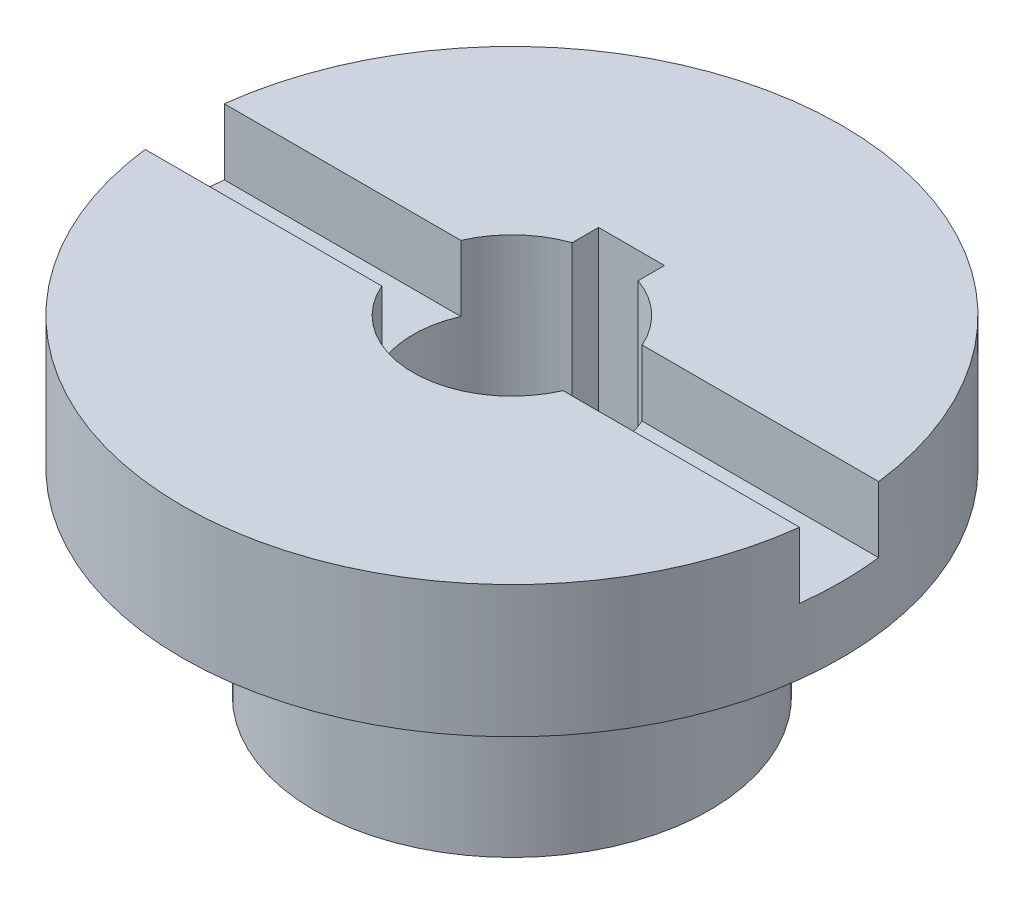
ISO-10303-21;
HEADER;
FILE_DESCRIPTION(('STEP AP214'),'2;1');
FILE_NAME('part.step','',(''),(''),'','','');
FILE_SCHEMA(('AUTOMOTIVE_DESIGN { 1 0 10303 214 1 1 1 1 }'));
ENDSEC;
DATA;
#1=APPLICATION_CONTEXT('core data for automotive mechanical design processes');
#2=APPLICATION_PROTOCOL_DEFINITION('international standard','automotive_design',2000,#1);
#3=PRODUCT_CONTEXT('',#1,'mechanical');
#4=PRODUCT('Part','Part','',(#3));
#5=PRODUCT_RELATED_PRODUCT_CATEGORY('part','',(#4));
#6=PRODUCT_DEFINITION_FORMATION('','',#4);
#7=PRODUCT_DEFINITION_CONTEXT('part definition',#1,'design');
#8=PRODUCT_DEFINITION('design','',#6,#7);
#9=PRODUCT_DEFINITION_SHAPE('','',#8);
#10=(LENGTH_UNIT() NAMED_UNIT(*) SI_UNIT(.MILLI.,.METRE.));
#11=(NAMED_UNIT(*) PLANE_ANGLE_UNIT() SI_UNIT($,.RADIAN.));
#12=(NAMED_UNIT(*) SI_UNIT($,.STERADIAN.) SOLID_ANGLE_UNIT());
#13=UNCERTAINTY_MEASURE_WITH_UNIT(LENGTH_MEASURE(1.E-05),#10,'distance_accuracy_value','');
#14=(GEOMETRIC_REPRESENTATION_CONTEXT(3) GLOBAL_UNCERTAINTY_ASSIGNED_CONTEXT((#13)) GLOBAL_UNIT_ASSIGNED_CONTEXT((#10,
#11,#12)) REPRESENTATION_CONTEXT('',''));
#15=CARTESIAN_POINT('',(0.,0.,0.));
#16=DIRECTION('',(0.,0.,1.));
#17=DIRECTION('',(1.,0.,0.));
#18=AXIS2_PLACEMENT_3D('',#15,#16,#17);
#19=CARTESIAN_POINT('',(0.,0.,0.));
#20=DIRECTION('',(0.,-1.,0.));
#21=DIRECTION('',(0.,0.,-1.));
#22=AXIS2_PLACEMENT_3D('',#19,#20,#21);
#23=PLANE('',#22);
#24=CARTESIAN_POINT('',(0.,0.,0.));
#25=DIRECTION('',(0.,1.,0.));
#26=DIRECTION('',(0.,0.,1.));
#27=AXIS2_PLACEMENT_3D('',#24,#25,#26);
#28=CIRCLE('',#27,50.);
#29=CARTESIAN_POINT('',(-49.6386945839634,0.,6.));
#30=VERTEX_POINT('',#29);
#31=CARTESIAN_POINT('',(49.6386945839634,0.,6.));
#32=VERTEX_POINT('',#31);
#33=EDGE_CURVE('E153',#30,#32,#28,.T.);
#34=ORIENTED_EDGE('',*,*,#33,.T.);
#35=DIRECTION('',(1.,0.,0.));
#36=VECTOR('',#35,1.);
#37=CARTESIAN_POINT('',(-59.6876701786652,0.,6.));
#38=LINE('',#37,#36);
#39=CARTESIAN_POINT('',(13.7477270848675,0.,6.));
#40=VERTEX_POINT('',#39);
#41=EDGE_CURVE('E144',#40,#32,#38,.T.);
#42=ORIENTED_EDGE('',*,*,#41,.F.);
#43=CARTESIAN_POINT('',(0.,0.,0.));
#44=DIRECTION('',(0.,1.,0.));
#45=DIRECTION('',(0.,0.,1.));
#46=AXIS2_PLACEMENT_3D('',#43,#44,#45);
#47=CIRCLE('',#46,15.);
#48=CARTESIAN_POINT('',(-13.7477270848675,0.,6.));
#49=VERTEX_POINT('',#48);
#50=EDGE_CURVE('E218',#49,#40,#47,.T.);
#51=ORIENTED_EDGE('',*,*,#50,.F.);
#52=EDGE_CURVE('E179',#30,#49,#38,.T.);
#53=ORIENTED_EDGE('',*,*,#52,.F.);
#54=EDGE_LOOP('',(#34,#42,#51,#53));
#55=FACE_BOUND('',#54,.T.);
#56=ADVANCED_FACE('F39',(#55),#23,.F.);
#57=CARTESIAN_POINT('',(49.6386945839634,0.,-6.));
#58=VERTEX_POINT('',#57);
#59=CARTESIAN_POINT('',(-49.6386945839634,0.,-6.));
#60=VERTEX_POINT('',#59);
#61=EDGE_CURVE('E142',#58,#60,#28,.T.);
#62=ORIENTED_EDGE('',*,*,#61,.T.);
#63=DIRECTION('',(-1.,0.,0.));
#64=VECTOR('',#63,1.);
#65=CARTESIAN_POINT('',(-59.6876701786652,0.,-6.));
#66=LINE('',#65,#64);
#67=CARTESIAN_POINT('',(-13.7477270848675,0.,-6.));
#68=VERTEX_POINT('',#67);
#69=EDGE_CURVE('E148',#68,#60,#66,.T.);
#70=ORIENTED_EDGE('',*,*,#69,.F.);
#71=CARTESIAN_POINT('',(-5.,0.,-14.142135623731));
#72=VERTEX_POINT('',#71);
#73=EDGE_CURVE('E203',#72,#68,#47,.T.);
#74=ORIENTED_EDGE('',*,*,#73,.F.);
#75=DIRECTION('',(0.,0.,1.));
#76=VECTOR('',#75,1.);
#77=CARTESIAN_POINT('',(-5.,0.,-14.142135623731));
#78=LINE('',#77,#76);
#79=CARTESIAN_POINT('',(-5.,0.,-18.142135623731));
#80=VERTEX_POINT('',#79);
#81=EDGE_CURVE('E214',#80,#72,#78,.T.);
#82=ORIENTED_EDGE('',*,*,#81,.F.);
#83=DIRECTION('',(-1.,0.,0.));
#84=VECTOR('',#83,1.);
#85=CARTESIAN_POINT('',(-5.,0.,-18.142135623731));
#86=LINE('',#85,#84);
#87=CARTESIAN_POINT('',(5.,0.,-18.142135623731));
#88=VERTEX_POINT('',#87);
#89=EDGE_CURVE('E215',#88,#80,#86,.T.);
#90=ORIENTED_EDGE('',*,*,#89,.F.);
#91=DIRECTION('',(0.,0.,-1.));
#92=VECTOR('',#91,1.);
#93=CARTESIAN_POINT('',(5.,0.,-14.142135623731));
#94=LINE('',#93,#92);
#95=CARTESIAN_POINT('',(4.99999999999999,0.,-14.142135623731));
#96=VERTEX_POINT('',#95);
#97=EDGE_CURVE('E198',#96,#88,#94,.T.);
#98=ORIENTED_EDGE('',*,*,#97,.F.);
#99=CARTESIAN_POINT('',(13.7477270848675,0.,-6.));
#100=VERTEX_POINT('',#99);
#101=EDGE_CURVE('E145',#100,#96,#47,.T.);
#102=ORIENTED_EDGE('',*,*,#101,.F.);
#103=EDGE_CURVE('E128',#58,#100,#66,.T.);
#104=ORIENTED_EDGE('',*,*,#103,.F.);
#105=EDGE_LOOP('',(#62,#70,#74,#82,#90,#98,#102,#104));
#106=FACE_BOUND('',#105,.T.);
#107=ADVANCED_FACE('F41',(#106),#23,.F.);
#108=CARTESIAN_POINT('',(0.,54.1187739463601,0.));
#109=DIRECTION('',(0.,1.,0.));
#110=DIRECTION('',(0.,0.,1.));
#111=AXIS2_PLACEMENT_3D('',#108,#109,#110);
#112=CYLINDRICAL_SURFACE('',#111,50.);
#113=CARTESIAN_POINT('',(0.,-10.,0.));
#114=DIRECTION('',(0.,-1.,0.));
#115=DIRECTION('',(0.,0.,-1.));
#116=AXIS2_PLACEMENT_3D('',#113,#114,#115);
#117=CIRCLE('',#116,50.);
#118=CARTESIAN_POINT('',(49.6386945839634,-10.,-6.));
#119=VERTEX_POINT('',#118);
#120=CARTESIAN_POINT('',(49.6386945839634,-10.,6.));
#121=VERTEX_POINT('',#120);
#122=EDGE_CURVE('E138',#119,#121,#117,.T.);
#123=ORIENTED_EDGE('',*,*,#122,.T.);
#124=DIRECTION('',(0.,1.,0.));
#125=VECTOR('',#124,1.);
#126=CARTESIAN_POINT('',(49.6386945839634,54.1187739463601,6.));
#127=LINE('',#126,#125);
#128=EDGE_CURVE('E191',#121,#32,#127,.T.);
#129=ORIENTED_EDGE('',*,*,#128,.T.);
#130=ORIENTED_EDGE('',*,*,#33,.F.);
#131=DIRECTION('',(0.,1.,0.));
#132=VECTOR('',#131,1.);
#133=CARTESIAN_POINT('',(-49.6386945839634,54.1187739463601,6.));
#134=LINE('',#133,#132);
#135=CARTESIAN_POINT('',(-49.6386945839634,-10.,6.));
#136=VERTEX_POINT('',#135);
#137=EDGE_CURVE('E187',#30,#136,#134,.F.);
#138=ORIENTED_EDGE('',*,*,#137,.T.);
#139=CARTESIAN_POINT('',(-49.6386945839634,-10.,-6.));
#140=VERTEX_POINT('',#139);
#141=EDGE_CURVE('E186',#136,#140,#117,.T.);
#142=ORIENTED_EDGE('',*,*,#141,.T.);
#143=DIRECTION('',(0.,1.,0.));
#144=VECTOR('',#143,1.);
#145=CARTESIAN_POINT('',(-49.6386945839634,54.1187739463601,-6.));
#146=LINE('',#145,#144);
#147=EDGE_CURVE('E132',#140,#60,#146,.T.);
#148=ORIENTED_EDGE('',*,*,#147,.T.);
#149=ORIENTED_EDGE('',*,*,#61,.F.);
#150=DIRECTION('',(0.,1.,0.));
#151=VECTOR('',#150,1.);
#152=CARTESIAN_POINT('',(49.6386945839634,54.1187739463601,-6.));
#153=LINE('',#152,#151);
#154=EDGE_CURVE('E130',#58,#119,#153,.F.);
#155=ORIENTED_EDGE('',*,*,#154,.T.);
#156=EDGE_LOOP('',(#123,#129,#130,#138,#142,#148,#149,#155));
#157=FACE_BOUND('',#156,.T.);
#158=CARTESIAN_POINT('',(0.,-20.,0.));
#159=DIRECTION('',(0.,1.,0.));
#160=DIRECTION('',(0.,0.,1.));
#161=AXIS2_PLACEMENT_3D('',#158,#159,#160);
#162=CIRCLE('',#161,50.);
#163=CARTESIAN_POINT('',(0.,-20.,50.));
#164=VERTEX_POINT('',#163);
#165=EDGE_CURVE('E159',#164,#164,#162,.T.);
#166=ORIENTED_EDGE('',*,*,#165,.T.);
#167=EDGE_LOOP('',(#166));
#168=FACE_BOUND('',#167,.T.);
#169=ADVANCED_FACE('F149',(#157,#168),#112,.T.);
#170=CARTESIAN_POINT('',(50.,-20.,0.));
#171=DIRECTION('',(0.,1.,0.));
#172=DIRECTION('',(0.,0.,1.));
#173=AXIS2_PLACEMENT_3D('',#170,#171,#172);
#174=PLANE('',#173);
#175=ORIENTED_EDGE('',*,*,#165,.F.);
#176=EDGE_LOOP('',(#175));
#177=FACE_BOUND('',#176,.T.);
#178=CARTESIAN_POINT('',(0.,-20.,0.));
#179=DIRECTION('',(0.,1.,0.));
#180=DIRECTION('',(0.,0.,1.));
#181=AXIS2_PLACEMENT_3D('',#178,#179,#180);
#182=CIRCLE('',#181,33.);
#183=CARTESIAN_POINT('',(0.,-20.,33.));
#184=VERTEX_POINT('',#183);
#185=EDGE_CURVE('E232',#184,#184,#182,.T.);
#186=ORIENTED_EDGE('',*,*,#185,.T.);
#187=EDGE_LOOP('',(#186));
#188=FACE_BOUND('',#187,.T.);
#189=ADVANCED_FACE('F244',(#177,#188),#174,.F.);
#190=CARTESIAN_POINT('',(0.,-23.,0.));
#191=DIRECTION('',(0.,1.,0.));
#192=DIRECTION('',(0.,0.,1.));
#193=AXIS2_PLACEMENT_3D('',#190,#191,#192);
#194=TOROIDAL_SURFACE('',#193,33.,3.);
#195=ORIENTED_EDGE('',*,*,#185,.F.);
#196=EDGE_LOOP('',(#195));
#197=FACE_BOUND('',#196,.T.);
#198=CARTESIAN_POINT('',(0.,-23.,0.));
#199=DIRECTION('',(0.,1.,0.));
#200=DIRECTION('',(0.,0.,1.));
#201=AXIS2_PLACEMENT_3D('',#198,#199,#200);
#202=CIRCLE('',#201,30.);
#203=CARTESIAN_POINT('',(0.,-23.,30.));
#204=VERTEX_POINT('',#203);
#205=EDGE_CURVE('E235',#204,#204,#202,.T.);
#206=ORIENTED_EDGE('',*,*,#205,.T.);
#207=EDGE_LOOP('',(#206));
#208=FACE_BOUND('',#207,.T.);
#209=ADVANCED_FACE('F245',(#197,#208),#194,.F.);
#210=CARTESIAN_POINT('',(0.,54.1187739463601,0.));
#211=DIRECTION('',(0.,1.,0.));
#212=DIRECTION('',(0.,0.,1.));
#213=AXIS2_PLACEMENT_3D('',#210,#211,#212);
#214=CYLINDRICAL_SURFACE('',#213,30.);
#215=ORIENTED_EDGE('',*,*,#205,.F.);
#216=EDGE_LOOP('',(#215));
#217=FACE_BOUND('',#216,.T.);
#218=CARTESIAN_POINT('',(0.,-50.,0.));
#219=DIRECTION('',(0.,1.,0.));
#220=DIRECTION('',(0.,0.,1.));
#221=AXIS2_PLACEMENT_3D('',#218,#219,#220);
#222=CIRCLE('',#221,30.);
#223=CARTESIAN_POINT('',(0.,-50.,30.));
#224=VERTEX_POINT('',#223);
#225=EDGE_CURVE('E224',#224,#224,#222,.T.);
#226=ORIENTED_EDGE('',*,*,#225,.T.);
#227=EDGE_LOOP('',(#226));
#228=FACE_BOUND('',#227,.T.);
#229=ADVANCED_FACE('F246',(#217,#228),#214,.T.);
#230=CARTESIAN_POINT('',(30.,-50.,0.));
#231=DIRECTION('',(0.,1.,0.));
#232=DIRECTION('',(0.,0.,1.));
#233=AXIS2_PLACEMENT_3D('',#230,#231,#232);
#234=PLANE('',#233);
#235=CARTESIAN_POINT('',(0.,-50.,0.));
#236=DIRECTION('',(0.,1.,0.));
#237=DIRECTION('',(0.,0.,1.));
#238=AXIS2_PLACEMENT_3D('',#235,#236,#237);
#239=CIRCLE('',#238,15.);
#240=CARTESIAN_POINT('',(-5.,-50.,-14.142135623731));
#241=VERTEX_POINT('',#240);
#242=CARTESIAN_POINT('',(4.99999999999999,-50.,-14.142135623731));
#243=VERTEX_POINT('',#242);
#244=EDGE_CURVE('E210',#241,#243,#239,.T.);
#245=ORIENTED_EDGE('',*,*,#244,.T.);
#246=DIRECTION('',(0.,0.,-1.));
#247=VECTOR('',#246,1.);
#248=CARTESIAN_POINT('',(5.,-50.,-14.142135623731));
#249=LINE('',#248,#247);
#250=CARTESIAN_POINT('',(5.,-50.,-18.142135623731));
#251=VERTEX_POINT('',#250);
#252=EDGE_CURVE('E197',#243,#251,#249,.T.);
#253=ORIENTED_EDGE('',*,*,#252,.T.);
#254=DIRECTION('',(-1.,0.,0.));
#255=VECTOR('',#254,1.);
#256=CARTESIAN_POINT('',(-5.,-50.,-18.142135623731));
#257=LINE('',#256,#255);
#258=CARTESIAN_POINT('',(-5.,-50.,-18.142135623731));
#259=VERTEX_POINT('',#258);
#260=EDGE_CURVE('E199',#251,#259,#257,.T.);
#261=ORIENTED_EDGE('',*,*,#260,.T.);
#262=DIRECTION('',(0.,0.,1.));
#263=VECTOR('',#262,1.);
#264=CARTESIAN_POINT('',(-5.,-50.,-14.142135623731));
#265=LINE('',#264,#263);
#266=EDGE_CURVE('E204',#259,#241,#265,.T.);
#267=ORIENTED_EDGE('',*,*,#266,.T.);
#268=EDGE_LOOP('',(#245,#253,#261,#267));
#269=FACE_BOUND('',#268,.T.);
#270=ORIENTED_EDGE('',*,*,#225,.F.);
#271=EDGE_LOOP('',(#270));
#272=FACE_BOUND('',#271,.T.);
#273=ADVANCED_FACE('F280',(#269,#272),#234,.F.);
#274=CARTESIAN_POINT('',(5.,-50.,-14.142135623731));
#275=DIRECTION('',(1.,0.,0.));
#276=DIRECTION('',(0.,0.,-1.));
#277=AXIS2_PLACEMENT_3D('',#274,#275,#276);
#278=PLANE('',#277);
#279=ORIENTED_EDGE('',*,*,#97,.T.);
#280=DIRECTION('',(0.,1.,0.));
#281=VECTOR('',#280,1.);
#282=CARTESIAN_POINT('',(5.,-50.,-18.142135623731));
#283=LINE('',#282,#281);
#284=EDGE_CURVE('E209',#251,#88,#283,.T.);
#285=ORIENTED_EDGE('',*,*,#284,.F.);
#286=ORIENTED_EDGE('',*,*,#252,.F.);
#287=DIRECTION('',(0.,1.,0.));
#288=VECTOR('',#287,1.);
#289=CARTESIAN_POINT('',(4.99999999999999,-50.,-14.142135623731));
#290=LINE('',#289,#288);
#291=EDGE_CURVE('E219',#243,#96,#290,.T.);
#292=ORIENTED_EDGE('',*,*,#291,.T.);
#293=EDGE_LOOP('',(#279,#285,#286,#292));
#294=FACE_BOUND('',#293,.T.);
#295=ADVANCED_FACE('F268',(#294),#278,.F.);
#296=CARTESIAN_POINT('',(0.,-50.,0.));
#297=DIRECTION('',(0.,1.,0.));
#298=DIRECTION('',(0.,0.,1.));
#299=AXIS2_PLACEMENT_3D('',#296,#297,#298);
#300=CYLINDRICAL_SURFACE('',#299,15.);
#301=CARTESIAN_POINT('',(0.,-10.,0.));
#302=DIRECTION('',(0.,-1.,0.));
#303=DIRECTION('',(0.,0.,-1.));
#304=AXIS2_PLACEMENT_3D('',#301,#302,#303);
#305=CIRCLE('',#304,15.);
#306=CARTESIAN_POINT('',(-13.7477270848675,-10.,-6.));
#307=VERTEX_POINT('',#306);
#308=CARTESIAN_POINT('',(-13.7477270848675,-10.,6.));
#309=VERTEX_POINT('',#308);
#310=EDGE_CURVE('E158',#307,#309,#305,.F.);
#311=ORIENTED_EDGE('',*,*,#310,.T.);
#312=DIRECTION('',(0.,1.,0.));
#313=VECTOR('',#312,1.);
#314=CARTESIAN_POINT('',(-13.7477270848675,-50.,6.));
#315=LINE('',#314,#313);
#316=EDGE_CURVE('E11',#309,#49,#315,.T.);
#317=ORIENTED_EDGE('',*,*,#316,.T.);
#318=ORIENTED_EDGE('',*,*,#50,.T.);
#319=DIRECTION('',(0.,1.,0.));
#320=VECTOR('',#319,1.);
#321=CARTESIAN_POINT('',(13.7477270848675,-50.,6.));
#322=LINE('',#321,#320);
#323=CARTESIAN_POINT('',(13.7477270848675,-10.,6.));
#324=VERTEX_POINT('',#323);
#325=EDGE_CURVE('E164',#40,#324,#322,.F.);
#326=ORIENTED_EDGE('',*,*,#325,.T.);
#327=CARTESIAN_POINT('',(13.7477270848675,-10.,-6.));
#328=VERTEX_POINT('',#327);
#329=EDGE_CURVE('E155',#324,#328,#305,.F.);
#330=ORIENTED_EDGE('',*,*,#329,.T.);
#331=DIRECTION('',(0.,1.,0.));
#332=VECTOR('',#331,1.);
#333=CARTESIAN_POINT('',(13.7477270848675,-50.,-6.));
#334=LINE('',#333,#332);
#335=EDGE_CURVE('E156',#328,#100,#334,.T.);
#336=ORIENTED_EDGE('',*,*,#335,.T.);
#337=ORIENTED_EDGE('',*,*,#101,.T.);
#338=ORIENTED_EDGE('',*,*,#291,.F.);
#339=ORIENTED_EDGE('',*,*,#244,.F.);
#340=DIRECTION('',(0.,1.,0.));
#341=VECTOR('',#340,1.);
#342=CARTESIAN_POINT('',(-5.,-50.,-14.142135623731));
#343=LINE('',#342,#341);
#344=EDGE_CURVE('E221',#241,#72,#343,.T.);
#345=ORIENTED_EDGE('',*,*,#344,.T.);
#346=ORIENTED_EDGE('',*,*,#73,.T.);
#347=DIRECTION('',(0.,1.,0.));
#348=VECTOR('',#347,1.);
#349=CARTESIAN_POINT('',(-13.7477270848675,-50.,-6.));
#350=LINE('',#349,#348);
#351=EDGE_CURVE('E50',#68,#307,#350,.F.);
#352=ORIENTED_EDGE('',*,*,#351,.T.);
#353=EDGE_LOOP('',(#311,#317,#318,#326,#330,#336,#337,#338,#339,#345,#346,#352));
#354=FACE_BOUND('',#353,.T.);
#355=ADVANCED_FACE('F174',(#354),#300,.F.);
#356=CARTESIAN_POINT('',(-5.,-50.,-14.142135623731));
#357=DIRECTION('',(-1.,0.,0.));
#358=DIRECTION('',(0.,0.,1.));
#359=AXIS2_PLACEMENT_3D('',#356,#357,#358);
#360=PLANE('',#359);
#361=ORIENTED_EDGE('',*,*,#81,.T.);
#362=ORIENTED_EDGE('',*,*,#344,.F.);
#363=ORIENTED_EDGE('',*,*,#266,.F.);
#364=DIRECTION('',(0.,1.,0.));
#365=VECTOR('',#364,1.);
#366=CARTESIAN_POINT('',(-5.,-50.,-18.142135623731));
#367=LINE('',#366,#365);
#368=EDGE_CURVE('E229',#259,#80,#367,.T.);
#369=ORIENTED_EDGE('',*,*,#368,.T.);
#370=EDGE_LOOP('',(#361,#362,#363,#369));
#371=FACE_BOUND('',#370,.T.);
#372=ADVANCED_FACE('F278',(#371),#360,.F.);
#373=CARTESIAN_POINT('',(-5.,-50.,-18.142135623731));
#374=DIRECTION('',(0.,0.,-1.));
#375=DIRECTION('',(-1.,0.,0.));
#376=AXIS2_PLACEMENT_3D('',#373,#374,#375);
#377=PLANE('',#376);
#378=ORIENTED_EDGE('',*,*,#89,.T.);
#379=ORIENTED_EDGE('',*,*,#368,.F.);
#380=ORIENTED_EDGE('',*,*,#260,.F.);
#381=ORIENTED_EDGE('',*,*,#284,.T.);
#382=EDGE_LOOP('',(#378,#379,#380,#381));
#383=FACE_BOUND('',#382,.T.);
#384=ADVANCED_FACE('F273',(#383),#377,.F.);
#385=CARTESIAN_POINT('',(0.,-10.,0.));
#386=DIRECTION('',(0.,-1.,0.));
#387=DIRECTION('',(0.,0.,-1.));
#388=AXIS2_PLACEMENT_3D('',#385,#386,#387);
#389=PLANE('',#388);
#390=DIRECTION('',(-1.,0.,0.));
#391=VECTOR('',#390,1.);
#392=CARTESIAN_POINT('',(-59.6876701786652,-10.,-6.));
#393=LINE('',#392,#391);
#394=EDGE_CURVE('E61',#119,#328,#393,.T.);
#395=ORIENTED_EDGE('',*,*,#394,.T.);
#396=ORIENTED_EDGE('',*,*,#329,.F.);
#397=DIRECTION('',(1.,0.,0.));
#398=VECTOR('',#397,1.);
#399=CARTESIAN_POINT('',(-59.6876701786652,-10.,6.));
#400=LINE('',#399,#398);
#401=EDGE_CURVE('E185',#324,#121,#400,.T.);
#402=ORIENTED_EDGE('',*,*,#401,.T.);
#403=ORIENTED_EDGE('',*,*,#122,.F.);
#404=EDGE_LOOP('',(#395,#396,#402,#403));
#405=FACE_BOUND('',#404,.T.);
#406=ADVANCED_FACE('F262',(#405),#389,.F.);
#407=CARTESIAN_POINT('',(-59.6876701786652,-10.,-6.));
#408=DIRECTION('',(0.,0.,-1.));
#409=DIRECTION('',(-1.,0.,0.));
#410=AXIS2_PLACEMENT_3D('',#407,#408,#409);
#411=PLANE('',#410);
#412=ORIENTED_EDGE('',*,*,#103,.T.);
#413=ORIENTED_EDGE('',*,*,#335,.F.);
#414=ORIENTED_EDGE('',*,*,#394,.F.);
#415=ORIENTED_EDGE('',*,*,#154,.F.);
#416=EDGE_LOOP('',(#412,#413,#414,#415));
#417=FACE_BOUND('',#416,.T.);
#418=ADVANCED_FACE('F129',(#417),#411,.F.);
#419=CARTESIAN_POINT('',(-59.6876701786652,-10.,6.));
#420=DIRECTION('',(0.,0.,1.));
#421=DIRECTION('',(1.,0.,0.));
#422=AXIS2_PLACEMENT_3D('',#419,#420,#421);
#423=PLANE('',#422);
#424=ORIENTED_EDGE('',*,*,#401,.F.);
#425=ORIENTED_EDGE('',*,*,#325,.F.);
#426=ORIENTED_EDGE('',*,*,#41,.T.);
#427=ORIENTED_EDGE('',*,*,#128,.F.);
#428=EDGE_LOOP('',(#424,#425,#426,#427));
#429=FACE_BOUND('',#428,.T.);
#430=ADVANCED_FACE('F263',(#429),#423,.F.);
#431=ORIENTED_EDGE('',*,*,#52,.T.);
#432=ORIENTED_EDGE('',*,*,#316,.F.);
#433=EDGE_CURVE('E53',#136,#309,#400,.T.);
#434=ORIENTED_EDGE('',*,*,#433,.F.);
#435=ORIENTED_EDGE('',*,*,#137,.F.);
#436=EDGE_LOOP('',(#431,#432,#434,#435));
#437=FACE_BOUND('',#436,.T.);
#438=ADVANCED_FACE('F357',(#437),#423,.F.);
#439=EDGE_CURVE('E180',#307,#140,#393,.T.);
#440=ORIENTED_EDGE('',*,*,#439,.F.);
#441=ORIENTED_EDGE('',*,*,#351,.F.);
#442=ORIENTED_EDGE('',*,*,#69,.T.);
#443=ORIENTED_EDGE('',*,*,#147,.F.);
#444=EDGE_LOOP('',(#440,#441,#442,#443));
#445=FACE_BOUND('',#444,.T.);
#446=ADVANCED_FACE('F177',(#445),#411,.F.);
#447=ORIENTED_EDGE('',*,*,#433,.T.);
#448=ORIENTED_EDGE('',*,*,#310,.F.);
#449=ORIENTED_EDGE('',*,*,#439,.T.);
#450=ORIENTED_EDGE('',*,*,#141,.F.);
#451=EDGE_LOOP('',(#447,#448,#449,#450));
#452=FACE_BOUND('',#451,.T.);
#453=ADVANCED_FACE('F178',(#452),#389,.F.);
#454=CLOSED_SHELL('',(#56,#107,#169,#189,#209,#229,#273,#295,#355,#372,#384,#406,#418,#430,#438,
#446,#453));
#455=MANIFOLD_SOLID_BREP('B2',#454);
#456=ADVANCED_BREP_SHAPE_REPRESENTATION('',(#18,#455),#14);
#457=SHAPE_DEFINITION_REPRESENTATION(#9,#456);
ENDSEC;
END-ISO-10303-21;
